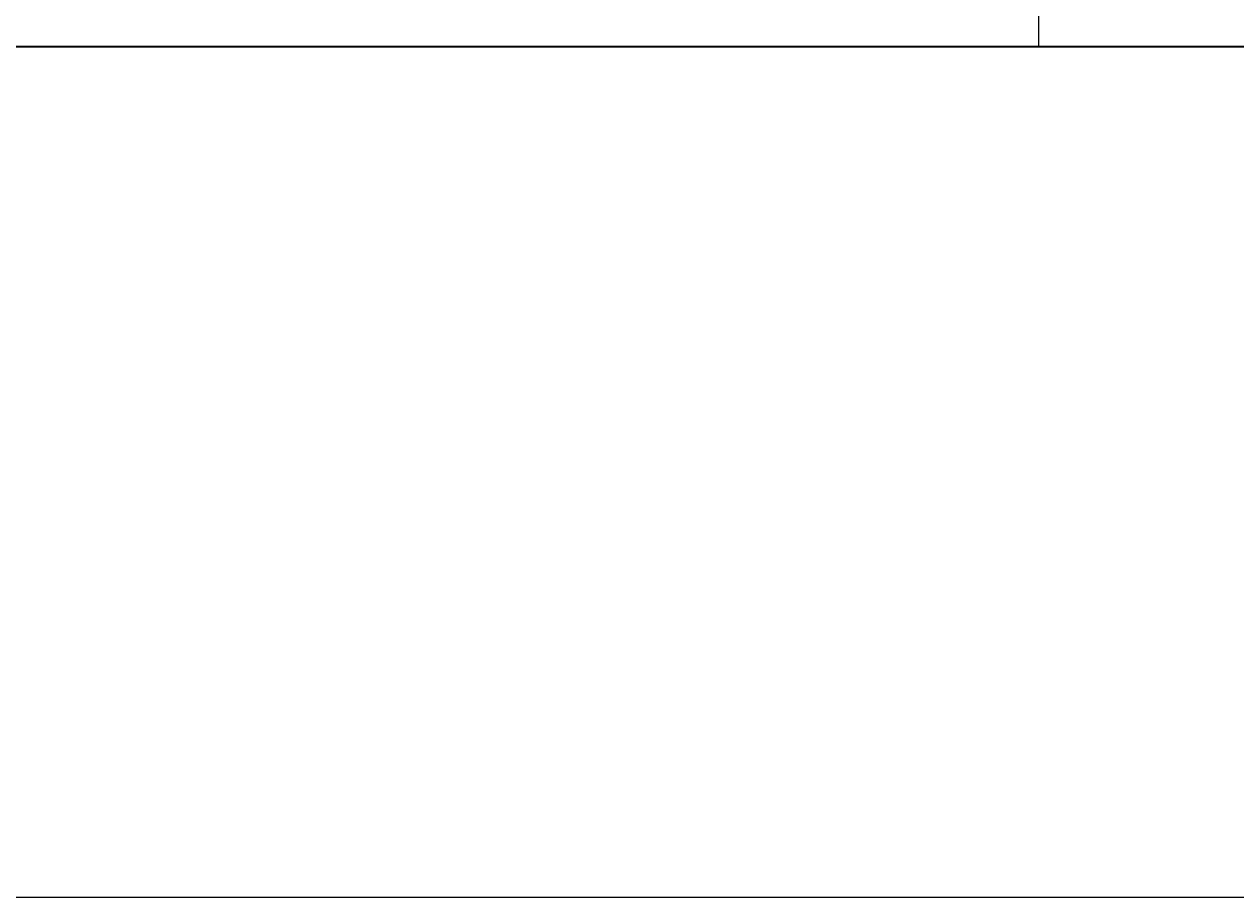
# Model space of a CAD drawing. Units: inches. Extents: x -61 to 1599, y -1316 to 257.
# Tile 157 of 204: x 1066 to 1214, y -1316 to -1208. Entities that reach past the tile are written whole.
import ezdxf

# ---------------------------------------------------------------- set-up
doc = ezdxf.new("R2010")
doc.units = ezdxf.units.IN
doc.header["$MEASUREMENT"] = 0
for name, color, linetype, lineweight in [('A-ANNO-DIMS', 2, 'Continuous', 18), ('WALLS', 4, 'Continuous', 35), ('WINDOWS', 220, 'Continuous', 18)]:
    doc.layers.add(name, color=color, linetype=linetype, lineweight=lineweight)
doc.styles.get("Standard").update_dxf_attribs({"font": 'arial.ttf'})
doc.dimstyles.get("Standard").update_dxf_attribs({"dimtxt": 0.18, "dimasz": 0.18, "dimexe": 0.18, "dimexo": 0.0625, "dimgap": 0.09, "dimtad": 0, "dimtih": 1, "dimtoh": 1, "dimdec": 0, "dimzin": 0, "dimdsep": 46, "dimlunit": 3, "dimtxsty": 'Standard', "dimcen": 0.09, "dimadec": 0, "dimazin": 0, "dimtfac": 1, "dimtdec": 0, "dimtofl": 0, "dimtmove": 0, "dimatfit": 3, "dimfxl": 1, "dimtolj": 1, "dimtzin": 0, "dimarcsym": 0})

# ---------------------------------------------------------------- blocks, each defined once
blk = doc.blocks.new('WIN-36IN-2')
for p, q in [((0, 9), (0, 0)), ((36, 9), (36, 0)), ((0, 5.26), (36, 5.26)), ((0, 4.5), (36, 4.5)), ((0, 4.5), (36, 4.5))]:
    blk.add_line(p, q)
blk = doc.blocks.new('*D690')
at = {"layer": 'A-ANNO-DIMS', "color": 0, "lineweight": -2, "transparency": 16777216}
for p, q in [((992.7, -1211.23), (992.7, -1315.72)), ((1522.7, -1211.23), (1522.7, -1315.72)), ((992.88, -1315.54), (1257.41, -1315.54)), ((1522.52, -1315.54), (1257.99, -1315.54))]:
    blk.add_line(p, q, dxfattribs=at)
at = {"layer": 'A-ANNO-DIMS', "color": 0, "transparency": 16777216}
for points in [[(992.88, -1315.51), (992.88, -1315.57), (992.7, -1315.54)], [(1522.52, -1315.51), (1522.52, -1315.57), (1522.7, -1315.54)]]:
    blk.add_solid(points, dxfattribs=at)
at = {"layer": 'DEFPOINTS', "color": 0, "transparency": 16777216}
for p in [(992.7, -1211.17), (1522.7, -1211.17), (1522.7, -1315.54)]:
    blk.add_point(p, dxfattribs=at)
at = {"layer": 'A-ANNO-DIMS', "color": 0, "transparency": 16777216, "insert": (1257.7, -1315.54), "char_height": 0.18, "attachment_point": 5}
blk.add_mtext('\\A1;530', dxfattribs=at)

msp = doc.modelspace()

# ---------------------------------------------------------------- linework, layer by layer
at = {"layer": 'WALLS'}
msp.add_line((992.7028, -1211.169), (1215.7028, -1211.169), dxfattribs=at)

# ---------------------------------------------------------------- block references
at = {"layer": 'WINDOWS'}
msp.add_blockref('WIN-36IN-2', (1190.158, -1211.1691), dxfattribs=at)

# ---------------------------------------------------------------- dimensions: what is measured, and where the dimension line sits
at = {"layer": 'A-ANNO-DIMS'}
dim = msp.add_linear_dim(base=(1522.7028, -1315.5446), p1=(992.7028, -1211.169), p2=(1522.7028, -1211.169), dimstyle='Standard', override={"dimdec": 0, "dimlfac": 1, "dimrnd": 0, "dimzin": 0, "dimdsep": 46, "dimlunit": 2}, dxfattribs=at)
dim.commit()
dim.dimension.update_dxf_attribs({"geometry": '*D690', "text_midpoint": (1257.7028, -1315.5446)})

doc.saveas('drawing.dxf')
